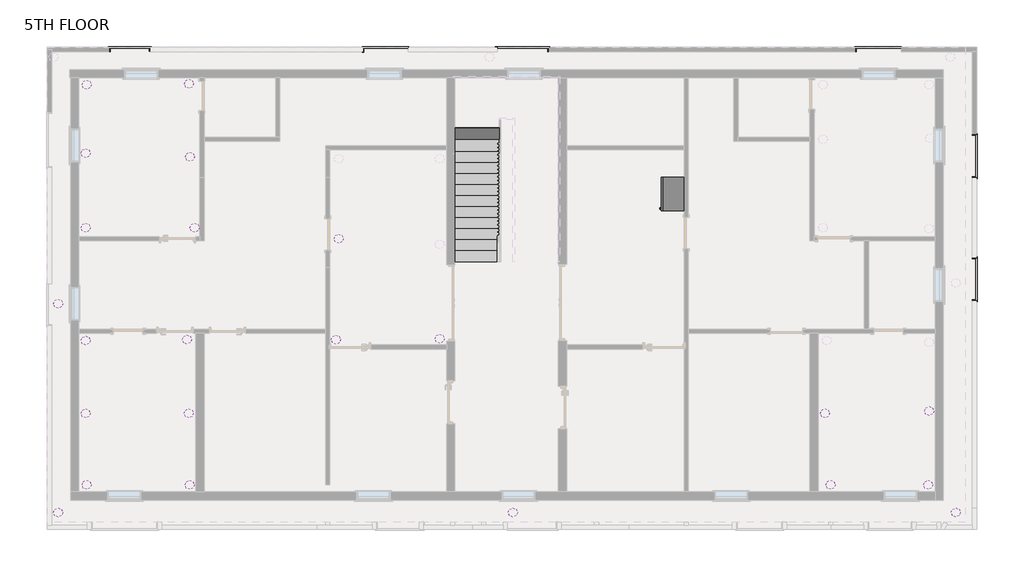
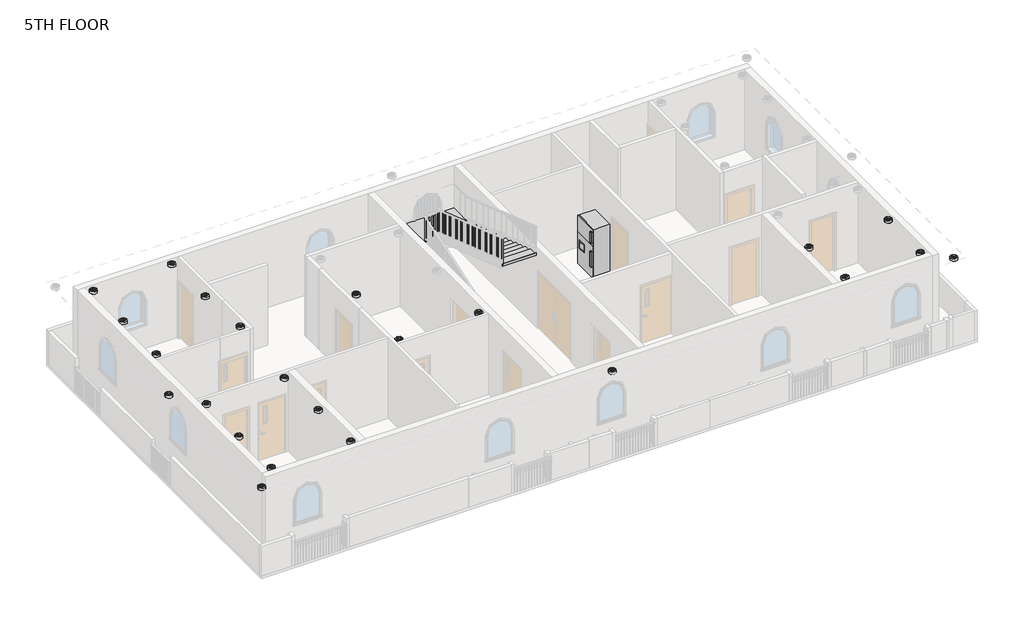
# One storey, part 6 of 7: 23 light fixtures, 6 railings, 1 furniture element, 1 stair flight.
"""IFC4 building model written with IfcOpenShell, lengths in millimetres."""

from ifc_helpers import new_model, si_unit, frame, origin, place, context, project, spatial, polyline, outline, extrude, faceted_brep, transform, mapped, element, save
from components import furniture_65fa61b5, ceiling_light_flat_round_60w_120v_7c4c2a52, stair_flight_d8047cd6

model = new_model("IFC4")

# Units and contexts
model_context = context("Model", 3, world=origin())
ifc_project = project(units=[si_unit("LENGTHUNIT", "METRE", prefix="MILLI")], contexts=[model_context])

# Site, building, storey
site = spatial("IfcSite", under=ifc_project)
building = spatial("IfcBuilding", under=site)
storey = spatial("IfcBuildingStorey", under=building, Name="5TH FLOOR", Elevation=16002.0)

# Furniture
placement = place(None, origin())
furniture_shape = furniture_65fa61b5(model_context)
element("IfcFurniture", 1, at=placement, inside=storey, context=model_context, shape_type="MappedRepresentation", body=[
    mapped(furniture_shape, transform((4507.551208, 3815.4567334, 16002.0), x_axis=(0.0, -1.0, 0.0), y_axis=(1.0, 0.0, 0.0), z_axis=(0.0, 0.0, 1.0))),
])

# Light fixtures
ceiling_light_flat_round_60w_120v_shape = ceiling_light_flat_round_60w_120v_7c4c2a52(model_context)
element("IfcLightFixture", 2, ObjectType="Ceiling Light - Flat Round : 60W - 120V", at=placement, inside=storey, context=model_context, shape_type="MappedRepresentation", body=[
    mapped(ceiling_light_flat_round_60w_120v_shape, transform((-12796.1987925, -4356.9932193, 16611.6), x_axis=(1.0, 0.0, 0.0), y_axis=(0.0, 1.0, 0.0), z_axis=(0.0, 0.0, 1.0))),
])
element("IfcLightFixture", 3, ObjectType="Ceiling Light - Flat Round : 60W - 120V", at=placement, inside=storey, context=model_context, shape_type="MappedRepresentation", body=[
    mapped(ceiling_light_flat_round_60w_120v_shape, transform((-249.1067989, -4356.9932193, 16611.6), x_axis=(1.0, 0.0, 0.0), y_axis=(0.0, 1.0, 0.0), z_axis=(0.0, 0.0, 1.0))),
])
element("IfcLightFixture", 4, ObjectType="Ceiling Light - Flat Round : 60W - 120V", at=placement, inside=storey, context=model_context, shape_type="MappedRepresentation", body=[
    mapped(ceiling_light_flat_round_60w_120v_shape, transform((11968.8012075, -4356.9932193, 16611.6), x_axis=(1.0, 0.0, 0.0), y_axis=(0.0, 1.0, 0.0), z_axis=(0.0, 0.0, 1.0))),
])
element("IfcLightFixture", 5, ObjectType="Ceiling Light - Flat Round : 60W - 120V", at=placement, inside=storey, context=model_context, shape_type="MappedRepresentation", body=[
    mapped(ceiling_light_flat_round_60w_120v_shape, transform((-12796.1987925, 1402.4567334, 16611.6), x_axis=(1.0, 0.0, 0.0), y_axis=(0.0, 1.0, 0.0), z_axis=(0.0, 0.0, 1.0))),
])
element("IfcLightFixture", 6, ObjectType="Ceiling Light - Flat Round : 60W - 120V", at=placement, inside=storey, context=model_context, shape_type="MappedRepresentation", body=[
    mapped(ceiling_light_flat_round_60w_120v_shape, transform((-12008.7987925, 7441.3067329, 16611.6), x_axis=(1.0, 0.0, 0.0), y_axis=(0.0, 1.0, 0.0), z_axis=(0.0, 0.0, 1.0))),
])
element("IfcLightFixture", 7, ObjectType="Ceiling Light - Flat Round : 60W - 120V", at=placement, inside=storey, context=model_context, shape_type="MappedRepresentation", body=[
    mapped(ceiling_light_flat_round_60w_120v_shape, transform((-9183.0487992, 7466.7067329, 16611.6), x_axis=(1.0, 0.0, 0.0), y_axis=(0.0, 1.0, 0.0), z_axis=(0.0, 0.0, 1.0))),
])
element("IfcLightFixture", 8, ObjectType="Ceiling Light - Flat Round : 60W - 120V", at=placement, inside=storey, context=model_context, shape_type="MappedRepresentation", body=[
    mapped(ceiling_light_flat_round_60w_120v_shape, transform((-12034.1987925, 3497.9567332, 16611.6), x_axis=(1.0, 0.0, 0.0), y_axis=(0.0, 1.0, 0.0), z_axis=(0.0, 0.0, 1.0))),
])
element("IfcLightFixture", 9, ObjectType="Ceiling Light - Flat Round : 60W - 120V", at=placement, inside=storey, context=model_context, shape_type="MappedRepresentation", body=[
    mapped(ceiling_light_flat_round_60w_120v_shape, transform((-9030.6487992, 3497.9567332, 16611.6), x_axis=(1.0, 0.0, 0.0), y_axis=(0.0, 1.0, 0.0), z_axis=(0.0, 0.0, 1.0))),
])
element("IfcLightFixture", 10, ObjectType="Ceiling Light - Flat Round : 60W - 120V", at=placement, inside=storey, context=model_context, shape_type="MappedRepresentation", body=[
    mapped(ceiling_light_flat_round_60w_120v_shape, transform((-12034.1987925, 386.4567334, 16611.6), x_axis=(1.0, 0.0, 0.0), y_axis=(0.0, 1.0, 0.0), z_axis=(0.0, 0.0, 1.0))),
])
element("IfcLightFixture", 11, ObjectType="Ceiling Light - Flat Round : 60W - 120V", at=placement, inside=storey, context=model_context, shape_type="MappedRepresentation", body=[
    mapped(ceiling_light_flat_round_60w_120v_shape, transform((-9240.1987992, 411.8567334, 16611.6), x_axis=(1.0, 0.0, 0.0), y_axis=(0.0, 1.0, 0.0), z_axis=(0.0, 0.0, 1.0))),
])
element("IfcLightFixture", 12, ObjectType="Ceiling Light - Flat Round : 60W - 120V", at=placement, inside=storey, context=model_context, shape_type="MappedRepresentation", body=[
    mapped(ceiling_light_flat_round_60w_120v_shape, transform((-12008.7987925, -3594.9932193, 16611.6), x_axis=(1.0, 0.0, 0.0), y_axis=(0.0, 1.0, 0.0), z_axis=(0.0, 0.0, 1.0))),
])
element("IfcLightFixture", 13, ObjectType="Ceiling Light - Flat Round : 60W - 120V", at=placement, inside=storey, context=model_context, shape_type="MappedRepresentation", body=[
    mapped(ceiling_light_flat_round_60w_120v_shape, transform((-9163.9987992, -3594.9932193, 16611.6), x_axis=(1.0, 0.0, 0.0), y_axis=(0.0, 1.0, 0.0), z_axis=(0.0, 0.0, 1.0))),
])
element("IfcLightFixture", 14, ObjectType="Ceiling Light - Flat Round : 60W - 120V", at=placement, inside=storey, context=model_context, shape_type="MappedRepresentation", body=[
    mapped(ceiling_light_flat_round_60w_120v_shape, transform((8514.4012079, -3594.9932193, 16611.6), x_axis=(1.0, 0.0, 0.0), y_axis=(0.0, 1.0, 0.0), z_axis=(0.0, 0.0, 1.0))),
])
element("IfcLightFixture", 15, ObjectType="Ceiling Light - Flat Round : 60W - 120V", at=placement, inside=storey, context=model_context, shape_type="MappedRepresentation", body=[
    mapped(ceiling_light_flat_round_60w_120v_shape, transform((11206.8012075, -3594.9932193, 16611.6), x_axis=(1.0, 0.0, 0.0), y_axis=(0.0, 1.0, 0.0), z_axis=(0.0, 0.0, 1.0))),
])
element("IfcLightFixture", 16, ObjectType="Ceiling Light - Flat Round : 60W - 120V", at=placement, inside=storey, context=model_context, shape_type="MappedRepresentation", body=[
    mapped(ceiling_light_flat_round_60w_120v_shape, transform((-5131.7487995, 408.4578621, 16611.6), x_axis=(1.0, 0.0, 0.0), y_axis=(0.0, 1.0, 0.0), z_axis=(0.0, 0.0, 1.0))),
])
element("IfcLightFixture", 17, ObjectType="Ceiling Light - Flat Round : 60W - 120V", at=placement, inside=storey, context=model_context, shape_type="MappedRepresentation", body=[
    mapped(ceiling_light_flat_round_60w_120v_shape, transform((-2267.8987998, 437.2567334, 16611.6), x_axis=(1.0, 0.0, 0.0), y_axis=(0.0, 1.0, 0.0), z_axis=(0.0, 0.0, 1.0))),
])
element("IfcLightFixture", 18, ObjectType="Ceiling Light - Flat Round : 60W - 120V", at=placement, inside=storey, context=model_context, shape_type="MappedRepresentation", body=[
    mapped(ceiling_light_flat_round_60w_120v_shape, transform((8362.0012079, -1623.5421379, 16611.6), x_axis=(1.0, 0.0, 0.0), y_axis=(0.0, 1.0, 0.0), z_axis=(0.0, 0.0, 1.0))),
])
element("IfcLightFixture", 19, ObjectType="Ceiling Light - Flat Round : 60W - 120V", at=placement, inside=storey, context=model_context, shape_type="MappedRepresentation", body=[
    mapped(ceiling_light_flat_round_60w_120v_shape, transform((11232.2012075, -1560.0808897, 16611.6), x_axis=(1.0, 0.0, 0.0), y_axis=(0.0, 1.0, 0.0), z_axis=(0.0, 0.0, 1.0))),
])
element("IfcLightFixture", 20, ObjectType="Ceiling Light - Flat Round : 60W - 120V", at=placement, inside=storey, context=model_context, shape_type="MappedRepresentation", body=[
    mapped(ceiling_light_flat_round_60w_120v_shape, transform((-5055.5487995, 3193.1567332, 16611.6), x_axis=(1.0, 0.0, 0.0), y_axis=(0.0, 1.0, 0.0), z_axis=(0.0, 0.0, 1.0))),
])
element("IfcLightFixture", 21, ObjectType="Ceiling Light - Flat Round : 60W - 120V", at=placement, inside=storey, context=model_context, shape_type="MappedRepresentation", body=[
    mapped(ceiling_light_flat_round_60w_120v_shape, transform((-12034.1987925, -1623.5421379, 16611.6), x_axis=(1.0, 0.0, 0.0), y_axis=(0.0, 1.0, 0.0), z_axis=(0.0, 0.0, 1.0))),
])
element("IfcLightFixture", 22, ObjectType="Ceiling Light - Flat Round : 60W - 120V", at=placement, inside=storey, context=model_context, shape_type="MappedRepresentation", body=[
    mapped(ceiling_light_flat_round_60w_120v_shape, transform((-9189.3987992, -1623.5421379, 16611.6), x_axis=(1.0, 0.0, 0.0), y_axis=(0.0, 1.0, 0.0), z_axis=(0.0, 0.0, 1.0))),
])
element("IfcLightFixture", 23, ObjectType="Ceiling Light - Flat Round : 60W - 120V", at=placement, inside=storey, context=model_context, shape_type="MappedRepresentation", body=[
    mapped(ceiling_light_flat_round_60w_120v_shape, transform((-12034.1987925, 5555.3567329, 16611.6), x_axis=(1.0, 0.0, 0.0), y_axis=(0.0, 1.0, 0.0), z_axis=(0.0, 0.0, 1.0))),
])
element("IfcLightFixture", 24, ObjectType="Ceiling Light - Flat Round : 60W - 120V", at=placement, inside=storey, context=model_context, shape_type="MappedRepresentation", body=[
    mapped(ceiling_light_flat_round_60w_120v_shape, transform((-9157.6487992, 5453.7567329, 16611.6), x_axis=(1.0, 0.0, 0.0), y_axis=(0.0, 1.0, 0.0), z_axis=(0.0, 0.0, 1.0))),
])

# Railings
element("IfcRailing", 25, ObjectType="Handrail - Rectangular", at=placement, inside=storey, context=model_context, shape_type="SolidModel", body=[
    faceted_brep([(-11412.4067989, 8355.7067329, 16916.4), (-11412.4067989, 8355.7067329, 16865.6), (-11361.6067989, 8355.7067329, 16865.6), (-11361.6067989, 8355.7067329, 16916.4), (-11412.4067989, 8495.4067329, 16916.4), (-11412.4067989, 8495.4067329, 16865.6), (-11361.6067989, 8444.6067329, 16865.6), (-11361.6067989, 8444.6067329, 16916.4), (-10231.3067989, 8495.4067329, 16916.4), (-10231.3067989, 8495.4067329, 16865.6), (-10282.1067989, 8444.6067329, 16865.6), (-10282.1067989, 8444.6067329, 16916.4), (-10231.3067989, 8368.4067329, 16916.4), (-10282.1067989, 8368.4067329, 16916.4), (-10282.1067989, 8368.4067329, 16865.6), (-10231.3067989, 8368.4067329, 16865.6)], [[[0, 1, 2, 3]], [[1, 0, 4, 5]], [[2, 1, 5, 6]], [[3, 2, 6, 7]], [[0, 3, 7, 4]], [[5, 4, 8, 9]], [[6, 5, 9, 10]], [[7, 6, 10, 11]], [[4, 7, 11, 8]], [[12, 13, 14, 15]], [[9, 8, 12, 15]], [[10, 9, 15, 14]], [[11, 10, 14, 13]], [[8, 11, 13, 12]]]),
    extrude(outline(polyline([(-10278.9317989, 8460.4817329), (-10278.9317989, 8479.5317329), (-10259.8817989, 8479.5317329), (-10259.8817989, 8460.4817329), (-10278.9317989, 8460.4817329)])), frame((0.0, 0.0, 16002.0), z_axis=(0.0, 0.0, 1.0), x_axis=(1.0, 0.0, 0.0)), (0.0, 0.0, 1.0), 863.6),
    extrude(outline(polyline([(-10380.5317989, 8460.4817329), (-10380.5317989, 8479.5317329), (-10361.4817989, 8479.5317329), (-10361.4817989, 8460.4817329), (-10380.5317989, 8460.4817329)])), frame((0.0, 0.0, 16002.0), z_axis=(0.0, 0.0, 1.0), x_axis=(1.0, 0.0, 0.0)), (0.0, 0.0, 1.0), 863.6),
    extrude(outline(polyline([(-10482.1317989, 8460.4817329), (-10482.1317989, 8479.5317329), (-10463.0817989, 8479.5317329), (-10463.0817989, 8460.4817329), (-10482.1317989, 8460.4817329)])), frame((0.0, 0.0, 16002.0), z_axis=(0.0, 0.0, 1.0), x_axis=(1.0, 0.0, 0.0)), (0.0, 0.0, 1.0), 863.6),
    extrude(outline(polyline([(-10583.7317989, 8460.4817329), (-10583.7317989, 8479.5317329), (-10564.6817989, 8479.5317329), (-10564.6817989, 8460.4817329), (-10583.7317989, 8460.4817329)])), frame((0.0, 0.0, 16002.0), z_axis=(0.0, 0.0, 1.0), x_axis=(1.0, 0.0, 0.0)), (0.0, 0.0, 1.0), 863.6),
    extrude(outline(polyline([(-10685.3317989, 8460.4817329), (-10685.3317989, 8479.5317329), (-10666.2817989, 8479.5317329), (-10666.2817989, 8460.4817329), (-10685.3317989, 8460.4817329)])), frame((0.0, 0.0, 16002.0), z_axis=(0.0, 0.0, 1.0), x_axis=(1.0, 0.0, 0.0)), (0.0, 0.0, 1.0), 863.6),
    extrude(outline(polyline([(-10786.9317989, 8460.4817329), (-10786.9317989, 8479.5317329), (-10767.8817989, 8479.5317329), (-10767.8817989, 8460.4817329), (-10786.9317989, 8460.4817329)])), frame((0.0, 0.0, 16002.0), z_axis=(0.0, 0.0, 1.0), x_axis=(1.0, 0.0, 0.0)), (0.0, 0.0, 1.0), 863.6),
    extrude(outline(polyline([(-10888.5317989, 8460.4817329), (-10888.5317989, 8479.5317329), (-10869.4817989, 8479.5317329), (-10869.4817989, 8460.4817329), (-10888.5317989, 8460.4817329)])), frame((0.0, 0.0, 16002.0), z_axis=(0.0, 0.0, 1.0), x_axis=(1.0, 0.0, 0.0)), (0.0, 0.0, 1.0), 863.6),
    extrude(outline(polyline([(-10990.1317989, 8460.4817329), (-10990.1317989, 8479.5317329), (-10971.0817989, 8479.5317329), (-10971.0817989, 8460.4817329), (-10990.1317989, 8460.4817329)])), frame((0.0, 0.0, 16002.0), z_axis=(0.0, 0.0, 1.0), x_axis=(1.0, 0.0, 0.0)), (0.0, 0.0, 1.0), 863.6),
    extrude(outline(polyline([(-11091.7317989, 8460.4817329), (-11091.7317989, 8479.5317329), (-11072.6817989, 8479.5317329), (-11072.6817989, 8460.4817329), (-11091.7317989, 8460.4817329)])), frame((0.0, 0.0, 16002.0), z_axis=(0.0, 0.0, 1.0), x_axis=(1.0, 0.0, 0.0)), (0.0, 0.0, 1.0), 863.6),
    extrude(outline(polyline([(-11193.3317989, 8460.4817329), (-11193.3317989, 8479.5317329), (-11174.2817989, 8479.5317329), (-11174.2817989, 8460.4817329), (-11193.3317989, 8460.4817329)])), frame((0.0, 0.0, 16002.0), z_axis=(0.0, 0.0, 1.0), x_axis=(1.0, 0.0, 0.0)), (0.0, 0.0, 1.0), 863.6),
    extrude(outline(polyline([(-11294.9317989, 8460.4817329), (-11294.9317989, 8479.5317329), (-11275.8817989, 8479.5317329), (-11275.8817989, 8460.4817329), (-11294.9317989, 8460.4817329)])), frame((0.0, 0.0, 16002.0), z_axis=(0.0, 0.0, 1.0), x_axis=(1.0, 0.0, 0.0)), (0.0, 0.0, 1.0), 863.6),
    extrude(outline(polyline([(-11377.4817989, 8447.7817329), (-11396.5317989, 8447.7817329), (-11396.5317989, 8466.8317329), (-11377.4817989, 8466.8317329), (-11377.4817989, 8447.7817329)])), frame((0.0, 0.0, 16002.0), z_axis=(0.0, 0.0, 1.0), x_axis=(1.0, 0.0, 0.0)), (0.0, 0.0, 1.0), 863.6),
    extrude(outline(polyline([(-10266.2317989, 8460.4817329), (-10266.2317989, 8479.5317329), (-10247.1817989, 8479.5317329), (-10247.1817989, 8460.4817329), (-10266.2317989, 8460.4817329)])), frame((0.0, 0.0, 16002.0), z_axis=(0.0, 0.0, 1.0), x_axis=(1.0, 0.0, 0.0)), (0.0, 0.0, 1.0), 863.6),
    extrude(outline(polyline([(-11377.4817989, 8460.4817329), (-11396.5317989, 8460.4817329), (-11396.5317989, 8479.5317329), (-11377.4817989, 8479.5317329), (-11377.4817989, 8460.4817329)])), frame((0.0, 0.0, 16002.0), z_axis=(0.0, 0.0, 1.0), x_axis=(1.0, 0.0, 0.0)), (0.0, 0.0, 1.0), 863.6),
    extrude(outline(polyline([(-10266.2317989, 8387.4567329), (-10247.1817989, 8387.4567329), (-10247.1817989, 8368.4067329), (-10266.2317989, 8368.4067329), (-10266.2317989, 8387.4567329)])), frame((0.0, 0.0, 16002.0), z_axis=(0.0, 0.0, 1.0), x_axis=(1.0, 0.0, 0.0)), (0.0, 0.0, 1.0), 863.6),
    extrude(outline(polyline([(-11377.4817989, 8355.7067329), (-11396.5317989, 8355.7067329), (-11396.5317989, 8374.7567329), (-11377.4817989, 8374.7567329), (-11377.4817989, 8355.7067329)])), frame((0.0, 0.0, 16002.0), z_axis=(0.0, 0.0, 1.0), x_axis=(1.0, 0.0, 0.0)), (0.0, 0.0, 1.0), 863.6),
])
element("IfcRailing", 26, ObjectType="Handrail - Rectangular", at=placement, inside=storey, context=model_context, shape_type="SolidModel", body=[
    faceted_brep([(-4407.8487992, 8336.6567329, 16916.4), (-4407.8487992, 8336.6567329, 16865.6), (-4357.0487992, 8336.6567329, 16865.6), (-4357.0487992, 8336.6567329, 16916.4), (-4407.8487992, 8495.4067329, 16916.4), (-4407.8487992, 8495.4067329, 16865.6), (-4357.0487992, 8444.6067329, 16865.6), (-4357.0487992, 8444.6067329, 16916.4), (-3120.4490672, 8495.4067329, 16916.4), (-3120.4490672, 8444.6067329, 16916.4), (-3120.4490672, 8444.6067329, 16865.6), (-3120.4490672, 8495.4067329, 16865.6)], [[[0, 1, 2, 3]], [[1, 0, 4, 5]], [[2, 1, 5, 6]], [[3, 2, 6, 7]], [[0, 3, 7, 4]], [[8, 9, 10, 11]], [[5, 4, 8, 11]], [[6, 5, 11, 10]], [[7, 6, 10, 9]], [[4, 7, 9, 8]]]),
    extrude(outline(polyline([(-3172.7737992, 8460.4817329), (-3172.7737992, 8479.5317329), (-3153.7237992, 8479.5317329), (-3153.7237992, 8460.4817329), (-3172.7737992, 8460.4817329)])), frame((0.0, 0.0, 16002.0), z_axis=(0.0, 0.0, 1.0), x_axis=(1.0, 0.0, 0.0)), (0.0, 0.0, 1.0), 863.6),
    extrude(outline(polyline([(-3274.3737992, 8460.4817329), (-3274.3737992, 8479.5317329), (-3255.3237992, 8479.5317329), (-3255.3237992, 8460.4817329), (-3274.3737992, 8460.4817329)])), frame((0.0, 0.0, 16002.0), z_axis=(0.0, 0.0, 1.0), x_axis=(1.0, 0.0, 0.0)), (0.0, 0.0, 1.0), 863.6),
    extrude(outline(polyline([(-3375.9737992, 8460.4817329), (-3375.9737992, 8479.5317329), (-3356.9237992, 8479.5317329), (-3356.9237992, 8460.4817329), (-3375.9737992, 8460.4817329)])), frame((0.0, 0.0, 16002.0), z_axis=(0.0, 0.0, 1.0), x_axis=(1.0, 0.0, 0.0)), (0.0, 0.0, 1.0), 863.6),
    extrude(outline(polyline([(-3477.5737992, 8460.4817329), (-3477.5737992, 8479.5317329), (-3458.5237992, 8479.5317329), (-3458.5237992, 8460.4817329), (-3477.5737992, 8460.4817329)])), frame((0.0, 0.0, 16002.0), z_axis=(0.0, 0.0, 1.0), x_axis=(1.0, 0.0, 0.0)), (0.0, 0.0, 1.0), 863.6),
    extrude(outline(polyline([(-3579.1737992, 8460.4817329), (-3579.1737992, 8479.5317329), (-3560.1237992, 8479.5317329), (-3560.1237992, 8460.4817329), (-3579.1737992, 8460.4817329)])), frame((0.0, 0.0, 16002.0), z_axis=(0.0, 0.0, 1.0), x_axis=(1.0, 0.0, 0.0)), (0.0, 0.0, 1.0), 863.6),
    extrude(outline(polyline([(-3680.7737992, 8460.4817329), (-3680.7737992, 8479.5317329), (-3661.7237992, 8479.5317329), (-3661.7237992, 8460.4817329), (-3680.7737992, 8460.4817329)])), frame((0.0, 0.0, 16002.0), z_axis=(0.0, 0.0, 1.0), x_axis=(1.0, 0.0, 0.0)), (0.0, 0.0, 1.0), 863.6),
    extrude(outline(polyline([(-3782.3737992, 8460.4817329), (-3782.3737992, 8479.5317329), (-3763.3237992, 8479.5317329), (-3763.3237992, 8460.4817329), (-3782.3737992, 8460.4817329)])), frame((0.0, 0.0, 16002.0), z_axis=(0.0, 0.0, 1.0), x_axis=(1.0, 0.0, 0.0)), (0.0, 0.0, 1.0), 863.6),
    extrude(outline(polyline([(-3883.9737992, 8460.4817329), (-3883.9737992, 8479.5317329), (-3864.9237992, 8479.5317329), (-3864.9237992, 8460.4817329), (-3883.9737992, 8460.4817329)])), frame((0.0, 0.0, 16002.0), z_axis=(0.0, 0.0, 1.0), x_axis=(1.0, 0.0, 0.0)), (0.0, 0.0, 1.0), 863.6),
    extrude(outline(polyline([(-3985.5737992, 8460.4817329), (-3985.5737992, 8479.5317329), (-3966.5237992, 8479.5317329), (-3966.5237992, 8460.4817329), (-3985.5737992, 8460.4817329)])), frame((0.0, 0.0, 16002.0), z_axis=(0.0, 0.0, 1.0), x_axis=(1.0, 0.0, 0.0)), (0.0, 0.0, 1.0), 863.6),
    extrude(outline(polyline([(-4087.1737992, 8460.4817329), (-4087.1737992, 8479.5317329), (-4068.1237992, 8479.5317329), (-4068.1237992, 8460.4817329), (-4087.1737992, 8460.4817329)])), frame((0.0, 0.0, 16002.0), z_axis=(0.0, 0.0, 1.0), x_axis=(1.0, 0.0, 0.0)), (0.0, 0.0, 1.0), 863.6),
    extrude(outline(polyline([(-4188.7737992, 8460.4817329), (-4188.7737992, 8479.5317329), (-4169.7237992, 8479.5317329), (-4169.7237992, 8460.4817329), (-4188.7737992, 8460.4817329)])), frame((0.0, 0.0, 16002.0), z_axis=(0.0, 0.0, 1.0), x_axis=(1.0, 0.0, 0.0)), (0.0, 0.0, 1.0), 863.6),
    extrude(outline(polyline([(-4290.3737992, 8460.4817329), (-4290.3737992, 8479.5317329), (-4271.3237992, 8479.5317329), (-4271.3237992, 8460.4817329), (-4290.3737992, 8460.4817329)])), frame((0.0, 0.0, 16002.0), z_axis=(0.0, 0.0, 1.0), x_axis=(1.0, 0.0, 0.0)), (0.0, 0.0, 1.0), 863.6),
    extrude(outline(polyline([(-4372.9237992, 8428.7317329), (-4391.9737992, 8428.7317329), (-4391.9737992, 8447.7817329), (-4372.9237992, 8447.7817329), (-4372.9237992, 8428.7317329)])), frame((0.0, 0.0, 16002.0), z_axis=(0.0, 0.0, 1.0), x_axis=(1.0, 0.0, 0.0)), (0.0, 0.0, 1.0), 863.6),
    extrude(outline(polyline([(-4372.9237992, 8460.4817329), (-4391.9737992, 8460.4817329), (-4391.9737992, 8479.5317329), (-4372.9237992, 8479.5317329), (-4372.9237992, 8460.4817329)])), frame((0.0, 0.0, 16002.0), z_axis=(0.0, 0.0, 1.0), x_axis=(1.0, 0.0, 0.0)), (0.0, 0.0, 1.0), 863.6),
    extrude(outline(polyline([(-3139.4990672, 8460.4817329), (-3139.4990672, 8479.5317329), (-3120.4490672, 8479.5317329), (-3120.4490672, 8460.4817329), (-3139.4990672, 8460.4817329)])), frame((0.0, 0.0, 16002.0), z_axis=(0.0, 0.0, 1.0), x_axis=(1.0, 0.0, 0.0)), (0.0, 0.0, 1.0), 863.6),
    extrude(outline(polyline([(-4372.9237992, 8336.6567329), (-4391.9737992, 8336.6567329), (-4391.9737992, 8355.7067329), (-4372.9237992, 8355.7067329), (-4372.9237992, 8336.6567329)])), frame((0.0, 0.0, 16002.0), z_axis=(0.0, 0.0, 1.0), x_axis=(1.0, 0.0, 0.0)), (0.0, 0.0, 1.0), 863.6),
])
element("IfcRailing", 27, ObjectType="Handrail - Rectangular", at=placement, inside=storey, context=model_context, shape_type="SolidModel", body=[
    faceted_brep([(-732.8490672, 8355.7067329, 16916.4), (-732.8490672, 8355.7067329, 16865.6), (-682.0490672, 8355.7067329, 16865.6), (-682.0490672, 8355.7067329, 16916.4), (-732.8490672, 8495.4067329, 16916.4), (-732.8490672, 8495.4067329, 16865.6), (-682.0490672, 8444.6067329, 16865.6), (-682.0490672, 8444.6067329, 16916.4), (766.8932011, 8495.4067329, 16916.4), (766.8932011, 8495.4067329, 16865.6), (716.0932011, 8444.6067329, 16865.6), (716.0932011, 8444.6067329, 16916.4), (766.8932011, 8355.7067329, 16916.4), (716.0932011, 8355.7067329, 16916.4), (716.0932011, 8355.7067329, 16865.6), (766.8932011, 8355.7067329, 16865.6)], [[[0, 1, 2, 3]], [[1, 0, 4, 5]], [[2, 1, 5, 6]], [[3, 2, 6, 7]], [[0, 3, 7, 4]], [[5, 4, 8, 9]], [[6, 5, 9, 10]], [[7, 6, 10, 11]], [[4, 7, 11, 8]], [[12, 13, 14, 15]], [[9, 8, 12, 15]], [[10, 9, 15, 14]], [[11, 10, 14, 13]], [[8, 11, 13, 12]]]),
    extrude(outline(polyline([(731.9682011, 8377.9317329), (751.0182011, 8377.9317329), (751.0182011, 8358.8817329), (731.9682011, 8358.8817329), (731.9682011, 8377.9317329)])), frame((0.0, 0.0, 16002.0), z_axis=(0.0, 0.0, 1.0), x_axis=(1.0, 0.0, 0.0)), (0.0, 0.0, 1.0), 863.6),
    extrude(outline(polyline([(705.4259328, 8460.4817329), (705.4259328, 8479.5317329), (724.4759328, 8479.5317329), (724.4759328, 8460.4817329), (705.4259328, 8460.4817329)])), frame((0.0, 0.0, 16002.0), z_axis=(0.0, 0.0, 1.0), x_axis=(1.0, 0.0, 0.0)), (0.0, 0.0, 1.0), 863.6),
    extrude(outline(polyline([(603.8259328, 8460.4817329), (603.8259328, 8479.5317329), (622.8759328, 8479.5317329), (622.8759328, 8460.4817329), (603.8259328, 8460.4817329)])), frame((0.0, 0.0, 16002.0), z_axis=(0.0, 0.0, 1.0), x_axis=(1.0, 0.0, 0.0)), (0.0, 0.0, 1.0), 863.6),
    extrude(outline(polyline([(502.2259328, 8460.4817329), (502.2259328, 8479.5317329), (521.2759328, 8479.5317329), (521.2759328, 8460.4817329), (502.2259328, 8460.4817329)])), frame((0.0, 0.0, 16002.0), z_axis=(0.0, 0.0, 1.0), x_axis=(1.0, 0.0, 0.0)), (0.0, 0.0, 1.0), 863.6),
    extrude(outline(polyline([(400.6259328, 8460.4817329), (400.6259328, 8479.5317329), (419.6759328, 8479.5317329), (419.6759328, 8460.4817329), (400.6259328, 8460.4817329)])), frame((0.0, 0.0, 16002.0), z_axis=(0.0, 0.0, 1.0), x_axis=(1.0, 0.0, 0.0)), (0.0, 0.0, 1.0), 863.6),
    extrude(outline(polyline([(299.0259328, 8460.4817329), (299.0259328, 8479.5317329), (318.0759328, 8479.5317329), (318.0759328, 8460.4817329), (299.0259328, 8460.4817329)])), frame((0.0, 0.0, 16002.0), z_axis=(0.0, 0.0, 1.0), x_axis=(1.0, 0.0, 0.0)), (0.0, 0.0, 1.0), 863.6),
    extrude(outline(polyline([(197.4259328, 8460.4817329), (197.4259328, 8479.5317329), (216.4759328, 8479.5317329), (216.4759328, 8460.4817329), (197.4259328, 8460.4817329)])), frame((0.0, 0.0, 16002.0), z_axis=(0.0, 0.0, 1.0), x_axis=(1.0, 0.0, 0.0)), (0.0, 0.0, 1.0), 863.6),
    extrude(outline(polyline([(95.8259328, 8460.4817329), (95.8259328, 8479.5317329), (114.8759328, 8479.5317329), (114.8759328, 8460.4817329), (95.8259328, 8460.4817329)])), frame((0.0, 0.0, 16002.0), z_axis=(0.0, 0.0, 1.0), x_axis=(1.0, 0.0, 0.0)), (0.0, 0.0, 1.0), 863.6),
    extrude(outline(polyline([(-5.7740672, 8460.4817329), (-5.7740672, 8479.5317329), (13.2759328, 8479.5317329), (13.2759328, 8460.4817329), (-5.7740672, 8460.4817329)])), frame((0.0, 0.0, 16002.0), z_axis=(0.0, 0.0, 1.0), x_axis=(1.0, 0.0, 0.0)), (0.0, 0.0, 1.0), 863.6),
    extrude(outline(polyline([(-107.3740672, 8460.4817329), (-107.3740672, 8479.5317329), (-88.3240672, 8479.5317329), (-88.3240672, 8460.4817329), (-107.3740672, 8460.4817329)])), frame((0.0, 0.0, 16002.0), z_axis=(0.0, 0.0, 1.0), x_axis=(1.0, 0.0, 0.0)), (0.0, 0.0, 1.0), 863.6),
    extrude(outline(polyline([(-208.9740672, 8460.4817329), (-208.9740672, 8479.5317329), (-189.9240672, 8479.5317329), (-189.9240672, 8460.4817329), (-208.9740672, 8460.4817329)])), frame((0.0, 0.0, 16002.0), z_axis=(0.0, 0.0, 1.0), x_axis=(1.0, 0.0, 0.0)), (0.0, 0.0, 1.0), 863.6),
    extrude(outline(polyline([(-310.5740672, 8460.4817329), (-310.5740672, 8479.5317329), (-291.5240672, 8479.5317329), (-291.5240672, 8460.4817329), (-310.5740672, 8460.4817329)])), frame((0.0, 0.0, 16002.0), z_axis=(0.0, 0.0, 1.0), x_axis=(1.0, 0.0, 0.0)), (0.0, 0.0, 1.0), 863.6),
    extrude(outline(polyline([(-412.1740672, 8460.4817329), (-412.1740672, 8479.5317329), (-393.1240672, 8479.5317329), (-393.1240672, 8460.4817329), (-412.1740672, 8460.4817329)])), frame((0.0, 0.0, 16002.0), z_axis=(0.0, 0.0, 1.0), x_axis=(1.0, 0.0, 0.0)), (0.0, 0.0, 1.0), 863.6),
    extrude(outline(polyline([(-513.7740672, 8460.4817329), (-513.7740672, 8479.5317329), (-494.7240672, 8479.5317329), (-494.7240672, 8460.4817329), (-513.7740672, 8460.4817329)])), frame((0.0, 0.0, 16002.0), z_axis=(0.0, 0.0, 1.0), x_axis=(1.0, 0.0, 0.0)), (0.0, 0.0, 1.0), 863.6),
    extrude(outline(polyline([(-615.3740672, 8460.4817329), (-615.3740672, 8479.5317329), (-596.3240672, 8479.5317329), (-596.3240672, 8460.4817329), (-615.3740672, 8460.4817329)])), frame((0.0, 0.0, 16002.0), z_axis=(0.0, 0.0, 1.0), x_axis=(1.0, 0.0, 0.0)), (0.0, 0.0, 1.0), 863.6),
    extrude(outline(polyline([(-697.9240672, 8447.7817329), (-716.9740672, 8447.7817329), (-716.9740672, 8466.8317329), (-697.9240672, 8466.8317329), (-697.9240672, 8447.7817329)])), frame((0.0, 0.0, 16002.0), z_axis=(0.0, 0.0, 1.0), x_axis=(1.0, 0.0, 0.0)), (0.0, 0.0, 1.0), 863.6),
    extrude(outline(polyline([(731.9682011, 8460.4817329), (731.9682011, 8479.5317329), (751.0182011, 8479.5317329), (751.0182011, 8460.4817329), (731.9682011, 8460.4817329)])), frame((0.0, 0.0, 16002.0), z_axis=(0.0, 0.0, 1.0), x_axis=(1.0, 0.0, 0.0)), (0.0, 0.0, 1.0), 863.6),
    extrude(outline(polyline([(-697.9240672, 8460.4817329), (-716.9740672, 8460.4817329), (-716.9740672, 8479.5317329), (-697.9240672, 8479.5317329), (-697.9240672, 8460.4817329)])), frame((0.0, 0.0, 16002.0), z_axis=(0.0, 0.0, 1.0), x_axis=(1.0, 0.0, 0.0)), (0.0, 0.0, 1.0), 863.6),
    extrude(outline(polyline([(731.9682011, 8374.7567329), (751.0182011, 8374.7567329), (751.0182011, 8355.7067329), (731.9682011, 8355.7067329), (731.9682011, 8374.7567329)])), frame((0.0, 0.0, 16002.0), z_axis=(0.0, 0.0, 1.0), x_axis=(1.0, 0.0, 0.0)), (0.0, 0.0, 1.0), 863.6),
    extrude(outline(polyline([(-697.9240672, 8355.7067329), (-716.9740672, 8355.7067329), (-716.9740672, 8374.7567329), (-697.9240672, 8374.7567329), (-697.9240672, 8355.7067329)])), frame((0.0, 0.0, 16002.0), z_axis=(0.0, 0.0, 1.0), x_axis=(1.0, 0.0, 0.0)), (0.0, 0.0, 1.0), 863.6),
])
element("IfcRailing", 28, ObjectType="Handrail - Rectangular", at=placement, inside=storey, context=model_context, shape_type="SolidModel", body=[
    faceted_brep([(9174.2932011, 8355.7067329, 16916.4), (9174.2932011, 8355.7067329, 16865.6), (9225.0932011, 8355.7067329, 16865.6), (9225.0932011, 8355.7067329, 16916.4), (9174.2932011, 8495.4067329, 16916.4), (9174.2932011, 8495.4067329, 16865.6), (9225.0932011, 8444.6067329, 16865.6), (9225.0932011, 8444.6067329, 16916.4), (10462.2009401, 8495.4067329, 16916.4), (10462.2009401, 8444.6067329, 16916.4), (10462.2009401, 8444.6067329, 16865.6), (10462.2009401, 8495.4067329, 16865.6)], [[[0, 1, 2, 3]], [[1, 0, 4, 5]], [[2, 1, 5, 6]], [[3, 2, 6, 7]], [[0, 3, 7, 4]], [[8, 9, 10, 11]], [[5, 4, 8, 11]], [[6, 5, 11, 10]], [[7, 6, 10, 9]], [[4, 7, 9, 8]]]),
    extrude(outline(polyline([(10409.3682011, 8460.4817329), (10409.3682011, 8479.5317329), (10428.4182011, 8479.5317329), (10428.4182011, 8460.4817329), (10409.3682011, 8460.4817329)])), frame((0.0, 0.0, 16002.0), z_axis=(0.0, 0.0, 1.0), x_axis=(1.0, 0.0, 0.0)), (0.0, 0.0, 1.0), 863.6),
    extrude(outline(polyline([(10307.7682011, 8460.4817329), (10307.7682011, 8479.5317329), (10326.8182011, 8479.5317329), (10326.8182011, 8460.4817329), (10307.7682011, 8460.4817329)])), frame((0.0, 0.0, 16002.0), z_axis=(0.0, 0.0, 1.0), x_axis=(1.0, 0.0, 0.0)), (0.0, 0.0, 1.0), 863.6),
    extrude(outline(polyline([(10206.1682011, 8460.4817329), (10206.1682011, 8479.5317329), (10225.2182011, 8479.5317329), (10225.2182011, 8460.4817329), (10206.1682011, 8460.4817329)])), frame((0.0, 0.0, 16002.0), z_axis=(0.0, 0.0, 1.0), x_axis=(1.0, 0.0, 0.0)), (0.0, 0.0, 1.0), 863.6),
    extrude(outline(polyline([(10104.5682011, 8460.4817329), (10104.5682011, 8479.5317329), (10123.6182011, 8479.5317329), (10123.6182011, 8460.4817329), (10104.5682011, 8460.4817329)])), frame((0.0, 0.0, 16002.0), z_axis=(0.0, 0.0, 1.0), x_axis=(1.0, 0.0, 0.0)), (0.0, 0.0, 1.0), 863.6),
    extrude(outline(polyline([(10002.9682011, 8460.4817329), (10002.9682011, 8479.5317329), (10022.0182011, 8479.5317329), (10022.0182011, 8460.4817329), (10002.9682011, 8460.4817329)])), frame((0.0, 0.0, 16002.0), z_axis=(0.0, 0.0, 1.0), x_axis=(1.0, 0.0, 0.0)), (0.0, 0.0, 1.0), 863.6),
    extrude(outline(polyline([(9901.3682011, 8460.4817329), (9901.3682011, 8479.5317329), (9920.4182011, 8479.5317329), (9920.4182011, 8460.4817329), (9901.3682011, 8460.4817329)])), frame((0.0, 0.0, 16002.0), z_axis=(0.0, 0.0, 1.0), x_axis=(1.0, 0.0, 0.0)), (0.0, 0.0, 1.0), 863.6),
    extrude(outline(polyline([(9799.7682011, 8460.4817329), (9799.7682011, 8479.5317329), (9818.8182011, 8479.5317329), (9818.8182011, 8460.4817329), (9799.7682011, 8460.4817329)])), frame((0.0, 0.0, 16002.0), z_axis=(0.0, 0.0, 1.0), x_axis=(1.0, 0.0, 0.0)), (0.0, 0.0, 1.0), 863.6),
    extrude(outline(polyline([(9698.1682011, 8460.4817329), (9698.1682011, 8479.5317329), (9717.2182011, 8479.5317329), (9717.2182011, 8460.4817329), (9698.1682011, 8460.4817329)])), frame((0.0, 0.0, 16002.0), z_axis=(0.0, 0.0, 1.0), x_axis=(1.0, 0.0, 0.0)), (0.0, 0.0, 1.0), 863.6),
    extrude(outline(polyline([(9596.5682011, 8460.4817329), (9596.5682011, 8479.5317329), (9615.6182011, 8479.5317329), (9615.6182011, 8460.4817329), (9596.5682011, 8460.4817329)])), frame((0.0, 0.0, 16002.0), z_axis=(0.0, 0.0, 1.0), x_axis=(1.0, 0.0, 0.0)), (0.0, 0.0, 1.0), 863.6),
    extrude(outline(polyline([(9494.9682011, 8460.4817329), (9494.9682011, 8479.5317329), (9514.0182011, 8479.5317329), (9514.0182011, 8460.4817329), (9494.9682011, 8460.4817329)])), frame((0.0, 0.0, 16002.0), z_axis=(0.0, 0.0, 1.0), x_axis=(1.0, 0.0, 0.0)), (0.0, 0.0, 1.0), 863.6),
    extrude(outline(polyline([(9393.3682011, 8460.4817329), (9393.3682011, 8479.5317329), (9412.4182011, 8479.5317329), (9412.4182011, 8460.4817329), (9393.3682011, 8460.4817329)])), frame((0.0, 0.0, 16002.0), z_axis=(0.0, 0.0, 1.0), x_axis=(1.0, 0.0, 0.0)), (0.0, 0.0, 1.0), 863.6),
    extrude(outline(polyline([(9291.7682011, 8460.4817329), (9291.7682011, 8479.5317329), (9310.8182011, 8479.5317329), (9310.8182011, 8460.4817329), (9291.7682011, 8460.4817329)])), frame((0.0, 0.0, 16002.0), z_axis=(0.0, 0.0, 1.0), x_axis=(1.0, 0.0, 0.0)), (0.0, 0.0, 1.0), 863.6),
    extrude(outline(polyline([(9209.2182011, 8447.7817329), (9190.1682011, 8447.7817329), (9190.1682011, 8466.8317329), (9209.2182011, 8466.8317329), (9209.2182011, 8447.7817329)])), frame((0.0, 0.0, 16002.0), z_axis=(0.0, 0.0, 1.0), x_axis=(1.0, 0.0, 0.0)), (0.0, 0.0, 1.0), 863.6),
    extrude(outline(polyline([(9209.2182011, 8460.4817329), (9190.1682011, 8460.4817329), (9190.1682011, 8479.5317329), (9209.2182011, 8479.5317329), (9209.2182011, 8460.4817329)])), frame((0.0, 0.0, 16002.0), z_axis=(0.0, 0.0, 1.0), x_axis=(1.0, 0.0, 0.0)), (0.0, 0.0, 1.0), 863.6),
    extrude(outline(polyline([(10443.1509401, 8460.4817329), (10443.1509401, 8479.5317329), (10462.2009401, 8479.5317329), (10462.2009401, 8460.4817329), (10443.1509401, 8460.4817329)])), frame((0.0, 0.0, 16002.0), z_axis=(0.0, 0.0, 1.0), x_axis=(1.0, 0.0, 0.0)), (0.0, 0.0, 1.0), 863.6),
    extrude(outline(polyline([(9209.2182011, 8355.7067329), (9190.1682011, 8355.7067329), (9190.1682011, 8374.7567329), (9209.2182011, 8374.7567329), (9209.2182011, 8355.7067329)])), frame((0.0, 0.0, 16002.0), z_axis=(0.0, 0.0, 1.0), x_axis=(1.0, 0.0, 0.0)), (0.0, 0.0, 1.0), 863.6),
])
element("IfcRailing", 29, ObjectType="Handrail - Rectangular", at=placement, inside=storey, context=model_context, shape_type="SolidModel", body=[
    faceted_brep([(12426.0012043, 2691.5067329, 16916.4), (12426.0012043, 2691.5067329, 16865.6), (12426.0012043, 2640.7067329, 16865.6), (12426.0012043, 2640.7067329, 16916.4), (12565.7012043, 2691.5067329, 16916.4), (12565.7012043, 2691.5067329, 16865.6), (12514.9012043, 2640.7067329, 16865.6), (12514.9012043, 2640.7067329, 16916.4), (12565.7012043, 1453.2567334, 16916.4), (12565.7012043, 1453.2567334, 16865.6), (12514.9012043, 1504.0567334, 16865.6), (12514.9012043, 1504.0567334, 16916.4), (12426.0012043, 1453.2567334, 16916.4), (12426.0012043, 1504.0567334, 16916.4), (12426.0012043, 1504.0567334, 16865.6), (12426.0012043, 1453.2567334, 16865.6)], [[[0, 1, 2, 3]], [[1, 0, 4, 5]], [[2, 1, 5, 6]], [[3, 2, 6, 7]], [[0, 3, 7, 4]], [[5, 4, 8, 9]], [[6, 5, 9, 10]], [[7, 6, 10, 11]], [[4, 7, 11, 8]], [[12, 13, 14, 15]], [[9, 8, 12, 15]], [[10, 9, 15, 14]], [[11, 10, 14, 13]], [[8, 11, 13, 12]]]),
    extrude(outline(polyline([(12448.2262043, 1488.1817334), (12448.2262043, 1469.1317334), (12429.1762043, 1469.1317334), (12429.1762043, 1488.1817334), (12448.2262043, 1488.1817334)])), frame((0.0, 0.0, 16002.0), z_axis=(0.0, 0.0, 1.0), x_axis=(1.0, 0.0, 0.0)), (0.0, 0.0, 1.0), 863.6),
    extrude(outline(polyline([(12530.7762043, 1558.0317329), (12549.8262043, 1558.0317329), (12549.8262043, 1538.9817329), (12530.7762043, 1538.9817329), (12530.7762043, 1558.0317329)])), frame((0.0, 0.0, 16002.0), z_axis=(0.0, 0.0, 1.0), x_axis=(1.0, 0.0, 0.0)), (0.0, 0.0, 1.0), 863.6),
    extrude(outline(polyline([(12530.7762043, 1659.6317329), (12549.8262043, 1659.6317329), (12549.8262043, 1640.5817329), (12530.7762043, 1640.5817329), (12530.7762043, 1659.6317329)])), frame((0.0, 0.0, 16002.0), z_axis=(0.0, 0.0, 1.0), x_axis=(1.0, 0.0, 0.0)), (0.0, 0.0, 1.0), 863.6),
    extrude(outline(polyline([(12530.7762043, 1761.2317329), (12549.8262043, 1761.2317329), (12549.8262043, 1742.1817329), (12530.7762043, 1742.1817329), (12530.7762043, 1761.2317329)])), frame((0.0, 0.0, 16002.0), z_axis=(0.0, 0.0, 1.0), x_axis=(1.0, 0.0, 0.0)), (0.0, 0.0, 1.0), 863.6),
    extrude(outline(polyline([(12530.7762043, 1862.8317329), (12549.8262043, 1862.8317329), (12549.8262043, 1843.7817329), (12530.7762043, 1843.7817329), (12530.7762043, 1862.8317329)])), frame((0.0, 0.0, 16002.0), z_axis=(0.0, 0.0, 1.0), x_axis=(1.0, 0.0, 0.0)), (0.0, 0.0, 1.0), 863.6),
    extrude(outline(polyline([(12530.7762043, 1964.4317329), (12549.8262043, 1964.4317329), (12549.8262043, 1945.3817329), (12530.7762043, 1945.3817329), (12530.7762043, 1964.4317329)])), frame((0.0, 0.0, 16002.0), z_axis=(0.0, 0.0, 1.0), x_axis=(1.0, 0.0, 0.0)), (0.0, 0.0, 1.0), 863.6),
    extrude(outline(polyline([(12530.7762043, 2066.0317329), (12549.8262043, 2066.0317329), (12549.8262043, 2046.9817329), (12530.7762043, 2046.9817329), (12530.7762043, 2066.0317329)])), frame((0.0, 0.0, 16002.0), z_axis=(0.0, 0.0, 1.0), x_axis=(1.0, 0.0, 0.0)), (0.0, 0.0, 1.0), 863.6),
    extrude(outline(polyline([(12530.7762043, 2167.6317329), (12549.8262043, 2167.6317329), (12549.8262043, 2148.5817329), (12530.7762043, 2148.5817329), (12530.7762043, 2167.6317329)])), frame((0.0, 0.0, 16002.0), z_axis=(0.0, 0.0, 1.0), x_axis=(1.0, 0.0, 0.0)), (0.0, 0.0, 1.0), 863.6),
    extrude(outline(polyline([(12530.7762043, 2269.2317329), (12549.8262043, 2269.2317329), (12549.8262043, 2250.1817329), (12530.7762043, 2250.1817329), (12530.7762043, 2269.2317329)])), frame((0.0, 0.0, 16002.0), z_axis=(0.0, 0.0, 1.0), x_axis=(1.0, 0.0, 0.0)), (0.0, 0.0, 1.0), 863.6),
    extrude(outline(polyline([(12530.7762043, 2370.8317329), (12549.8262043, 2370.8317329), (12549.8262043, 2351.7817329), (12530.7762043, 2351.7817329), (12530.7762043, 2370.8317329)])), frame((0.0, 0.0, 16002.0), z_axis=(0.0, 0.0, 1.0), x_axis=(1.0, 0.0, 0.0)), (0.0, 0.0, 1.0), 863.6),
    extrude(outline(polyline([(12530.7762043, 2472.4317329), (12549.8262043, 2472.4317329), (12549.8262043, 2453.3817329), (12530.7762043, 2453.3817329), (12530.7762043, 2472.4317329)])), frame((0.0, 0.0, 16002.0), z_axis=(0.0, 0.0, 1.0), x_axis=(1.0, 0.0, 0.0)), (0.0, 0.0, 1.0), 863.6),
    extrude(outline(polyline([(12530.7762043, 2574.0317329), (12549.8262043, 2574.0317329), (12549.8262043, 2554.9817329), (12530.7762043, 2554.9817329), (12530.7762043, 2574.0317329)])), frame((0.0, 0.0, 16002.0), z_axis=(0.0, 0.0, 1.0), x_axis=(1.0, 0.0, 0.0)), (0.0, 0.0, 1.0), 863.6),
    extrude(outline(polyline([(12518.0762043, 2656.5817329), (12518.0762043, 2675.6317329), (12537.1262043, 2675.6317329), (12537.1262043, 2656.5817329), (12518.0762043, 2656.5817329)])), frame((0.0, 0.0, 16002.0), z_axis=(0.0, 0.0, 1.0), x_axis=(1.0, 0.0, 0.0)), (0.0, 0.0, 1.0), 863.6),
    extrude(outline(polyline([(12530.7762043, 1488.1817334), (12549.8262043, 1488.1817334), (12549.8262043, 1469.1317334), (12530.7762043, 1469.1317334), (12530.7762043, 1488.1817334)])), frame((0.0, 0.0, 16002.0), z_axis=(0.0, 0.0, 1.0), x_axis=(1.0, 0.0, 0.0)), (0.0, 0.0, 1.0), 863.6),
    extrude(outline(polyline([(12530.7762043, 2656.5817329), (12530.7762043, 2675.6317329), (12549.8262043, 2675.6317329), (12549.8262043, 2656.5817329), (12530.7762043, 2656.5817329)])), frame((0.0, 0.0, 16002.0), z_axis=(0.0, 0.0, 1.0), x_axis=(1.0, 0.0, 0.0)), (0.0, 0.0, 1.0), 863.6),
    extrude(outline(polyline([(12445.0512043, 1488.1817334), (12445.0512043, 1469.1317334), (12426.0012043, 1469.1317334), (12426.0012043, 1488.1817334), (12445.0512043, 1488.1817334)])), frame((0.0, 0.0, 16002.0), z_axis=(0.0, 0.0, 1.0), x_axis=(1.0, 0.0, 0.0)), (0.0, 0.0, 1.0), 863.6),
    extrude(outline(polyline([(12426.0012043, 2656.5817329), (12426.0012043, 2675.6317329), (12445.0512043, 2675.6317329), (12445.0512043, 2656.5817329), (12426.0012043, 2656.5817329)])), frame((0.0, 0.0, 16002.0), z_axis=(0.0, 0.0, 1.0), x_axis=(1.0, 0.0, 0.0)), (0.0, 0.0, 1.0), 863.6),
])
element("IfcRailing", 30, ObjectType="Handrail - Rectangular", at=placement, inside=storey, context=model_context, shape_type="SolidModel", body=[
    faceted_brep([(12426.0012043, 6095.1067329, 16916.4), (12426.0012043, 6095.1067329, 16865.6), (12426.0012043, 6044.3067329, 16865.6), (12426.0012043, 6044.3067329, 16916.4), (12565.7012043, 6095.1067329, 16916.4), (12565.7012043, 6095.1067329, 16865.6), (12514.9012043, 6044.3067329, 16865.6), (12514.9012043, 6044.3067329, 16916.4), (12565.7012043, 4850.5067329, 16916.4), (12565.7012043, 4850.5067329, 16865.6), (12514.9012043, 4901.3067329, 16865.6), (12514.9012043, 4901.3067329, 16916.4), (12426.0012043, 4850.5067329, 16916.4), (12426.0012043, 4901.3067329, 16916.4), (12426.0012043, 4901.3067329, 16865.6), (12426.0012043, 4850.5067329, 16865.6)], [[[0, 1, 2, 3]], [[1, 0, 4, 5]], [[2, 1, 5, 6]], [[3, 2, 6, 7]], [[0, 3, 7, 4]], [[5, 4, 8, 9]], [[6, 5, 9, 10]], [[7, 6, 10, 11]], [[4, 7, 11, 8]], [[12, 13, 14, 15]], [[9, 8, 12, 15]], [[10, 9, 15, 14]], [[11, 10, 14, 13]], [[8, 11, 13, 12]]]),
    extrude(outline(polyline([(12448.2262043, 4885.4317329), (12448.2262043, 4866.3817329), (12429.1762043, 4866.3817329), (12429.1762043, 4885.4317329), (12448.2262043, 4885.4317329)])), frame((0.0, 0.0, 16002.0), z_axis=(0.0, 0.0, 1.0), x_axis=(1.0, 0.0, 0.0)), (0.0, 0.0, 1.0), 863.6),
    extrude(outline(polyline([(12530.7762043, 4961.6317329), (12549.8262043, 4961.6317329), (12549.8262043, 4942.5817329), (12530.7762043, 4942.5817329), (12530.7762043, 4961.6317329)])), frame((0.0, 0.0, 16002.0), z_axis=(0.0, 0.0, 1.0), x_axis=(1.0, 0.0, 0.0)), (0.0, 0.0, 1.0), 863.6),
    extrude(outline(polyline([(12530.7762043, 5063.2317329), (12549.8262043, 5063.2317329), (12549.8262043, 5044.1817329), (12530.7762043, 5044.1817329), (12530.7762043, 5063.2317329)])), frame((0.0, 0.0, 16002.0), z_axis=(0.0, 0.0, 1.0), x_axis=(1.0, 0.0, 0.0)), (0.0, 0.0, 1.0), 863.6),
    extrude(outline(polyline([(12530.7762043, 5164.8317329), (12549.8262043, 5164.8317329), (12549.8262043, 5145.7817329), (12530.7762043, 5145.7817329), (12530.7762043, 5164.8317329)])), frame((0.0, 0.0, 16002.0), z_axis=(0.0, 0.0, 1.0), x_axis=(1.0, 0.0, 0.0)), (0.0, 0.0, 1.0), 863.6),
    extrude(outline(polyline([(12530.7762043, 5266.4317329), (12549.8262043, 5266.4317329), (12549.8262043, 5247.3817329), (12530.7762043, 5247.3817329), (12530.7762043, 5266.4317329)])), frame((0.0, 0.0, 16002.0), z_axis=(0.0, 0.0, 1.0), x_axis=(1.0, 0.0, 0.0)), (0.0, 0.0, 1.0), 863.6),
    extrude(outline(polyline([(12530.7762043, 5368.0317329), (12549.8262043, 5368.0317329), (12549.8262043, 5348.9817329), (12530.7762043, 5348.9817329), (12530.7762043, 5368.0317329)])), frame((0.0, 0.0, 16002.0), z_axis=(0.0, 0.0, 1.0), x_axis=(1.0, 0.0, 0.0)), (0.0, 0.0, 1.0), 863.6),
    extrude(outline(polyline([(12530.7762043, 5469.6317329), (12549.8262043, 5469.6317329), (12549.8262043, 5450.5817329), (12530.7762043, 5450.5817329), (12530.7762043, 5469.6317329)])), frame((0.0, 0.0, 16002.0), z_axis=(0.0, 0.0, 1.0), x_axis=(1.0, 0.0, 0.0)), (0.0, 0.0, 1.0), 863.6),
    extrude(outline(polyline([(12530.7762043, 5571.2317329), (12549.8262043, 5571.2317329), (12549.8262043, 5552.1817329), (12530.7762043, 5552.1817329), (12530.7762043, 5571.2317329)])), frame((0.0, 0.0, 16002.0), z_axis=(0.0, 0.0, 1.0), x_axis=(1.0, 0.0, 0.0)), (0.0, 0.0, 1.0), 863.6),
    extrude(outline(polyline([(12530.7762043, 5672.8317329), (12549.8262043, 5672.8317329), (12549.8262043, 5653.7817329), (12530.7762043, 5653.7817329), (12530.7762043, 5672.8317329)])), frame((0.0, 0.0, 16002.0), z_axis=(0.0, 0.0, 1.0), x_axis=(1.0, 0.0, 0.0)), (0.0, 0.0, 1.0), 863.6),
    extrude(outline(polyline([(12530.7762043, 5774.4317329), (12549.8262043, 5774.4317329), (12549.8262043, 5755.3817329), (12530.7762043, 5755.3817329), (12530.7762043, 5774.4317329)])), frame((0.0, 0.0, 16002.0), z_axis=(0.0, 0.0, 1.0), x_axis=(1.0, 0.0, 0.0)), (0.0, 0.0, 1.0), 863.6),
    extrude(outline(polyline([(12530.7762043, 5876.0317329), (12549.8262043, 5876.0317329), (12549.8262043, 5856.9817329), (12530.7762043, 5856.9817329), (12530.7762043, 5876.0317329)])), frame((0.0, 0.0, 16002.0), z_axis=(0.0, 0.0, 1.0), x_axis=(1.0, 0.0, 0.0)), (0.0, 0.0, 1.0), 863.6),
    extrude(outline(polyline([(12530.7762043, 5977.6317329), (12549.8262043, 5977.6317329), (12549.8262043, 5958.5817329), (12530.7762043, 5958.5817329), (12530.7762043, 5977.6317329)])), frame((0.0, 0.0, 16002.0), z_axis=(0.0, 0.0, 1.0), x_axis=(1.0, 0.0, 0.0)), (0.0, 0.0, 1.0), 863.6),
    extrude(outline(polyline([(12518.0762043, 6060.1817329), (12518.0762043, 6079.2317329), (12537.1262043, 6079.2317329), (12537.1262043, 6060.1817329), (12518.0762043, 6060.1817329)])), frame((0.0, 0.0, 16002.0), z_axis=(0.0, 0.0, 1.0), x_axis=(1.0, 0.0, 0.0)), (0.0, 0.0, 1.0), 863.6),
    extrude(outline(polyline([(12530.7762043, 4885.4317329), (12549.8262043, 4885.4317329), (12549.8262043, 4866.3817329), (12530.7762043, 4866.3817329), (12530.7762043, 4885.4317329)])), frame((0.0, 0.0, 16002.0), z_axis=(0.0, 0.0, 1.0), x_axis=(1.0, 0.0, 0.0)), (0.0, 0.0, 1.0), 863.6),
    extrude(outline(polyline([(12530.7762043, 6060.1817329), (12530.7762043, 6079.2317329), (12549.8262043, 6079.2317329), (12549.8262043, 6060.1817329), (12530.7762043, 6060.1817329)])), frame((0.0, 0.0, 16002.0), z_axis=(0.0, 0.0, 1.0), x_axis=(1.0, 0.0, 0.0)), (0.0, 0.0, 1.0), 863.6),
    extrude(outline(polyline([(12445.0512043, 4885.4317329), (12445.0512043, 4866.3817329), (12426.0012043, 4866.3817329), (12426.0012043, 4885.4317329), (12445.0512043, 4885.4317329)])), frame((0.0, 0.0, 16002.0), z_axis=(0.0, 0.0, 1.0), x_axis=(1.0, 0.0, 0.0)), (0.0, 0.0, 1.0), 863.6),
    extrude(outline(polyline([(12426.0012043, 6060.1817329), (12426.0012043, 6079.2317329), (12445.0512043, 6079.2317329), (12445.0512043, 6060.1817329), (12426.0012043, 6060.1817329)])), frame((0.0, 0.0, 16002.0), z_axis=(0.0, 0.0, 1.0), x_axis=(1.0, 0.0, 0.0)), (0.0, 0.0, 1.0), 863.6),
])

# Stair flight
stair_flight_shape = stair_flight_d8047cd6(model_context)
element("IfcStairFlight", 31, ObjectType="2\" Tread 1\" Nosing 1/4\" Riser", at=placement, inside=storey, context=model_context, shape_type="MappedRepresentation", body=[
    mapped(stair_flight_shape, transform((0.0, 0.0, 0.0), x_axis=(1.0, 0.0, 0.0), y_axis=(0.0, 1.0, 0.0), z_axis=(0.0, 0.0, 1.0))),
])

save(model, "model.ifc")

# Revit data of these elements
# Type
#   Default Elevation = 0
# Type "Ceiling Light - Flat Round : 60W - 120V"
#   Lamp = "A-19"
#   Assembly Code = "D5020220"
#   Wattage = 60 W
#   built-in parameter 1150110 = 1 (stored number, unit not read)
#   built-in parameter 1114217 = 1 (stored number, unit not read)
#   built-in parameter 1150109 = 1 (stored number, unit not read)
#   built-in parameter 1150113 = 1 (stored number, unit not read)
#   built-in parameter 1150115 = 1 (stored number, unit not read)
#   built-in parameter 1150105 = 272.155 (stored number, unit not read)
#   Light Source Symbol Size = 2' - 0"
#   built-in parameter 1150112 = 1 (stored number, unit not read)
#   built-in parameter 1150114 = 1 (stored number, unit not read)
#   built-in parameter 1150107 = 2800 (stored number, unit not read)
#   built-in parameter 1150106 = 2.72155 (stored number, unit not read)
#   Emit from Circle Diameter = 0' - 10"
#   built-in parameter 1150104 = 1.32387 (stored number, unit not read)
#   Ballast Voltage = 120 V
#   built-in parameter 1114218 = 1 (stored number, unit not read)
#   built-in parameter 1150133 = 10 (stored number, unit not read)
#   Lumens = 855 lm
#   Apparent Load = 60 VA
#   built-in parameter 1150134 = 4
#   built-in parameter 1150137 = 1
#   Color Filter = 16777215
#   built-in parameter 1140040 [instance default] = 1
#   Ballast Number of Poles = 1
#   Light Box Material = Steel, Paint Finish, Dark Gray, Matte
#   Diffuser Material = Glass, White, High Luminance
#   Wattage Comments = ""
#   Emit Shape Visible in Rendering = no
#   Dimming Lamp Color Temperature Shift = (empty or 0)
#   Default Elevation = 0
# Type "Handrail - Rectangular"
#   Assembly Code = "C2010400"
#   built-in parameter 1008612 = 0.0416667 (stored number, unit not read)
#   built-in parameter 1008611 = 0.0416667 (stored number, unit not read)
#   built-in parameter 1008609 = 0.333333 (stored number, unit not read)
#   built-in parameter 1008604 = 0.166667 (stored number, unit not read)
#   built-in parameter 1008603 = 0.166667 (stored number, unit not read)
#   Railing Height = 3' - 0"
#   built-in parameter 1008630 = 2
#   built-in parameter 1008610 = 2
#   built-in parameter 1008618 = Baluster - Square : 3/4"
# Element 1 (IfcFurniture)
#   Phase Created = New Construction
#   Materials on its faces: "Default", "Default 3", "Default 2"
# Element 2 (IfcLightFixture, "Ceiling Light - Flat Round : 60W - 120V")
#   Mark = "139"
#   built-in parameter 1140040 = 1
#   Phase Created = New Construction
#   Materials on its faces: "Glass, White, High Luminance", "Steel, Paint Finish, Dark Gray, Matte"
# Element 3 (IfcLightFixture, "Ceiling Light - Flat Round : 60W - 120V")
#   Mark = "140"
#   built-in parameter 1140040 = 1
#   Phase Created = New Construction
#   Materials on its faces: "Glass, White, High Luminance", "Steel, Paint Finish, Dark Gray, Matte"
# Element 4 (IfcLightFixture, "Ceiling Light - Flat Round : 60W - 120V")
#   Mark = "141"
#   built-in parameter 1140040 = 1
#   Phase Created = New Construction
#   Materials on its faces: "Glass, White, High Luminance", "Steel, Paint Finish, Dark Gray, Matte"
# Element 5 (IfcLightFixture, "Ceiling Light - Flat Round : 60W - 120V")
#   Mark = "143"
#   built-in parameter 1140040 = 1
#   Phase Created = New Construction
#   Materials on its faces: "Glass, White, High Luminance", "Steel, Paint Finish, Dark Gray, Matte"
# Element 6 (IfcLightFixture, "Ceiling Light - Flat Round : 60W - 120V")
#   Mark = "144"
#   built-in parameter 1140040 = 1
#   Phase Created = New Construction
#   Materials on its faces: "Glass, White, High Luminance", "Steel, Paint Finish, Dark Gray, Matte"
# Element 7 (IfcLightFixture, "Ceiling Light - Flat Round : 60W - 120V")
#   Mark = "145"
#   built-in parameter 1140040 = 1
#   Phase Created = New Construction
#   Materials on its faces: "Glass, White, High Luminance", "Steel, Paint Finish, Dark Gray, Matte"
# Element 8 (IfcLightFixture, "Ceiling Light - Flat Round : 60W - 120V")
#   Mark = "146"
#   built-in parameter 1140040 = 1
#   Phase Created = New Construction
#   Materials on its faces: "Glass, White, High Luminance", "Steel, Paint Finish, Dark Gray, Matte"
# Element 9 (IfcLightFixture, "Ceiling Light - Flat Round : 60W - 120V")
#   Mark = "147"
#   built-in parameter 1140040 = 1
#   Phase Created = New Construction
#   Materials on its faces: "Glass, White, High Luminance", "Steel, Paint Finish, Dark Gray, Matte"
# Element 10 (IfcLightFixture, "Ceiling Light - Flat Round : 60W - 120V")
#   Mark = "148"
#   built-in parameter 1140040 = 1
#   Phase Created = New Construction
#   Materials on its faces: "Glass, White, High Luminance", "Steel, Paint Finish, Dark Gray, Matte"
# Element 11 (IfcLightFixture, "Ceiling Light - Flat Round : 60W - 120V")
#   Mark = "149"
#   built-in parameter 1140040 = 1
#   Phase Created = New Construction
#   Materials on its faces: "Glass, White, High Luminance", "Steel, Paint Finish, Dark Gray, Matte"
# Element 12 (IfcLightFixture, "Ceiling Light - Flat Round : 60W - 120V")
#   Mark = "150"
#   built-in parameter 1140040 = 1
#   Phase Created = New Construction
#   Materials on its faces: "Glass, White, High Luminance", "Steel, Paint Finish, Dark Gray, Matte"
# Element 13 (IfcLightFixture, "Ceiling Light - Flat Round : 60W - 120V")
#   Mark = "151"
#   built-in parameter 1140040 = 1
#   Phase Created = New Construction
#   Materials on its faces: "Glass, White, High Luminance", "Steel, Paint Finish, Dark Gray, Matte"
# Element 14 (IfcLightFixture, "Ceiling Light - Flat Round : 60W - 120V")
#   Mark = "158"
#   built-in parameter 1140040 = 1
#   Phase Created = New Construction
#   Materials on its faces: "Glass, White, High Luminance", "Steel, Paint Finish, Dark Gray, Matte"
# Element 15 (IfcLightFixture, "Ceiling Light - Flat Round : 60W - 120V")
#   Mark = "159"
#   built-in parameter 1140040 = 1
#   Phase Created = New Construction
#   Materials on its faces: "Glass, White, High Luminance", "Steel, Paint Finish, Dark Gray, Matte"
# Element 16 (IfcLightFixture, "Ceiling Light - Flat Round : 60W - 120V")
#   Mark = "162"
#   built-in parameter 1140040 = 1
#   Phase Created = New Construction
#   Materials on its faces: "Glass, White, High Luminance", "Steel, Paint Finish, Dark Gray, Matte"
# Element 17 (IfcLightFixture, "Ceiling Light - Flat Round : 60W - 120V")
#   Mark = "163"
#   built-in parameter 1140040 = 1
#   Phase Created = New Construction
#   Materials on its faces: "Glass, White, High Luminance", "Steel, Paint Finish, Dark Gray, Matte"
# Element 18 (IfcLightFixture, "Ceiling Light - Flat Round : 60W - 120V")
#   Mark = "164"
#   built-in parameter 1140040 = 1
#   Phase Created = New Construction
#   Materials on its faces: "Glass, White, High Luminance", "Steel, Paint Finish, Dark Gray, Matte"
# Element 19 (IfcLightFixture, "Ceiling Light - Flat Round : 60W - 120V")
#   Mark = "165"
#   built-in parameter 1140040 = 1
#   Phase Created = New Construction
#   Materials on its faces: "Glass, White, High Luminance", "Steel, Paint Finish, Dark Gray, Matte"
# Element 20 (IfcLightFixture, "Ceiling Light - Flat Round : 60W - 120V")
#   Mark = "168"
#   built-in parameter 1140040 = 1
#   Phase Created = New Construction
#   Materials on its faces: "Glass, White, High Luminance", "Steel, Paint Finish, Dark Gray, Matte"
# Element 21 (IfcLightFixture, "Ceiling Light - Flat Round : 60W - 120V")
#   Mark = "170"
#   built-in parameter 1140040 = 1
#   Phase Created = New Construction
